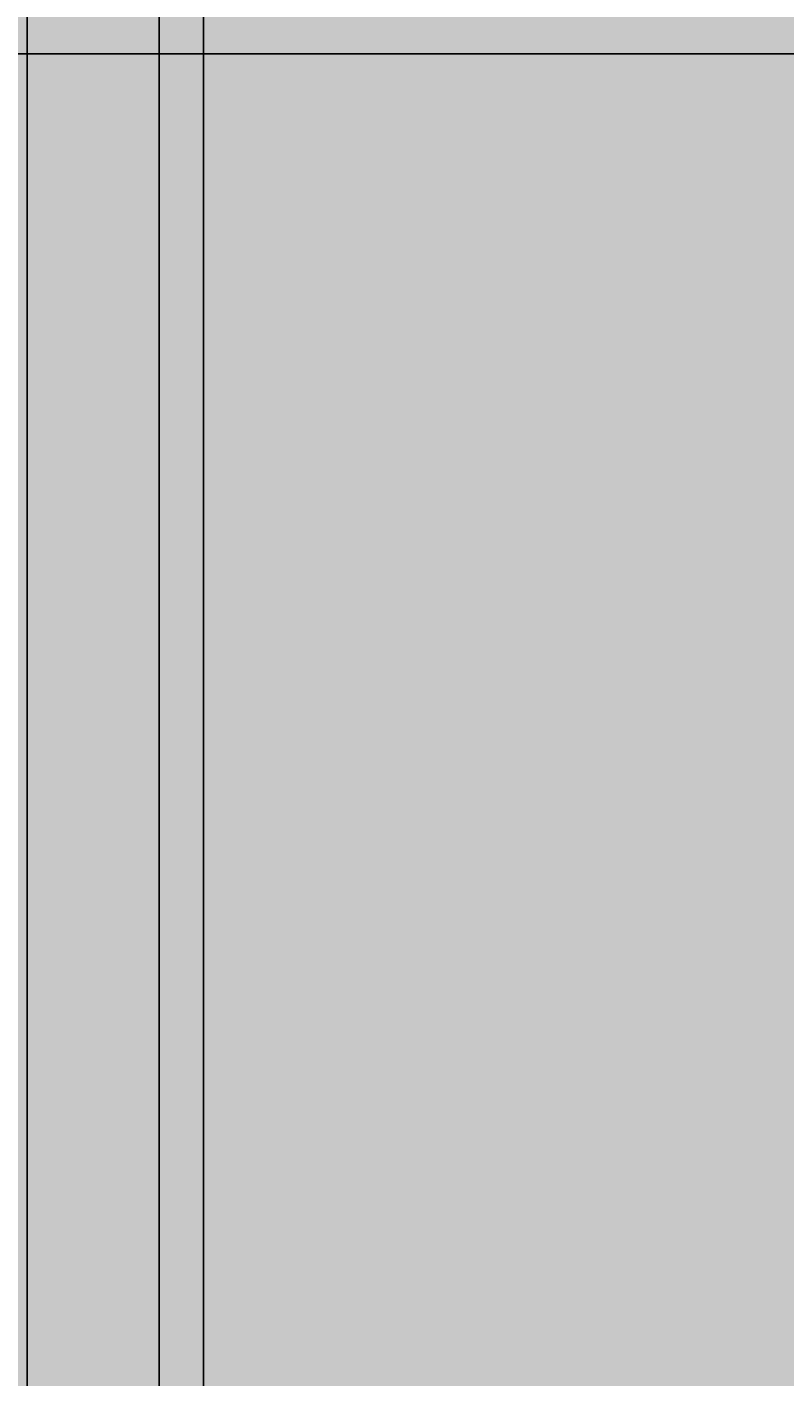
# Model space of a CAD drawing. Units: feet. Extents: x 2695 to 2912, y 795 to 1139.
# Tile 21 of 83: x 2774 to 2791, y 845 to 875. Entities that reach past the tile are written whole.
import ezdxf

# ---------------------------------------------------------------- set-up
doc = ezdxf.new("R2010")
doc.units = ezdxf.units.FT
for name, color, linetype, lineweight in [('A-ANNO-DIMS', 2, 'Continuous', 18), ('A-DOOR', 3, 'Continuous', 25), ('A-DOOR-PATT', 33, 'Continuous', 13), ('A-ELEV-PATT', 252, 'Continuous', 13)]:
    doc.layers.add(name, color=color, linetype=linetype, lineweight=lineweight)
doc.styles.get("Standard").update_dxf_attribs({"font": 'arial.ttf'})
doc.dimstyles.get("Standard").update_dxf_attribs({"dimtxt": 0.18, "dimasz": 0.18, "dimexe": 0.18, "dimexo": 0.0625, "dimgap": 0.09, "dimtad": 0, "dimtih": 1, "dimtoh": 1, "dimdec": 1, "dimzin": 0, "dimdsep": 46, "dimlunit": 3, "dimtxsty": 'Standard', "dimcen": 0.09, "dimadec": 0, "dimazin": 0, "dimtfac": 1, "dimtdec": 1, "dimtofl": 0, "dimtmove": 0, "dimatfit": 3, "dimfxl": 1, "dimtolj": 1, "dimtzin": 0, "dimarcsym": 0})

# ---------------------------------------------------------------- blocks, each defined once
blk = doc.blocks.new('*D13')
at = {"layer": 'A-ANNO-DIMS', "color": 0, "lineweight": -2, "transparency": 16777216}
for p, q in [((2758.214, 874.857), (2911.424, 874.857)), ((2911.244, 874.677), (2911.244, 843.076)), ((2911.244, 811.111), (2911.244, 842.712)), ((2890.699, 810.931), (2911.424, 810.931))]:
    blk.add_line(p, q, dxfattribs=at)
at = {"layer": 'A-ANNO-DIMS', "color": 0, "transparency": 16777216}
for points in [[(2911.214, 874.677), (2911.274, 874.677), (2911.244, 874.857)], [(2911.214, 811.111), (2911.274, 811.111), (2911.244, 810.931)]]:
    blk.add_solid(points, dxfattribs=at)
at = {"layer": 'Defpoints', "color": 0, "transparency": 16777216}
for p in [(2758.151, 874.857), (2911.244, 874.857), (2890.636, 810.931)]:
    blk.add_point(p, dxfattribs=at)
at = {"layer": 'A-ANNO-DIMS', "color": 0, "transparency": 16777216, "insert": (2911.244, 842.894), "char_height": 0.18, "attachment_point": 5}
blk.add_mtext('\\A1;63.93', dxfattribs=at)
blk = doc.blocks.new('*D14')
at = {"layer": 'A-ANNO-DIMS', "color": 0, "lineweight": -2, "transparency": 16777216}
for p, q in [((2838.439, 905.514), (2911.424, 905.514)), ((2911.244, 905.334), (2911.244, 890.368)), ((2911.244, 875.037), (2911.244, 890.004)), ((2758.214, 874.857), (2911.424, 874.857))]:
    blk.add_line(p, q, dxfattribs=at)
at = {"layer": 'A-ANNO-DIMS', "color": 0, "transparency": 16777216}
for points in [[(2911.214, 905.334), (2911.274, 905.334), (2911.244, 905.514)], [(2911.214, 875.037), (2911.274, 875.037), (2911.244, 874.857)]]:
    blk.add_solid(points, dxfattribs=at)
at = {"layer": 'Defpoints', "color": 0, "transparency": 16777216}
for p in [(2838.377, 905.514), (2911.244, 905.514), (2758.151, 874.857)]:
    blk.add_point(p, dxfattribs=at)
at = {"layer": 'A-ANNO-DIMS', "color": 0, "transparency": 16777216, "insert": (2911.244, 890.186), "char_height": 0.18, "attachment_point": 5}
blk.add_mtext('\\A1;30.66', dxfattribs=at)

msp = doc.modelspace()

# ---------------------------------------------------------------- hatches: boundary and pattern name
at = {"layer": 'A-DOOR-PATT'}
h = msp.add_hatch(color=256, dxfattribs=at)
h.set_gradient(color1=(211, 185, 150), color2=(211, 185, 150))
h.paths.add_polyline_path([(2805.9398, 905.5143), (2773.5029, 905.5143), (2773.5029, 810.9306), (2776.4999, 810.9306), (2776.4999, 902.5174), (2802.9429, 902.5174), (2802.9429, 810.9306), (2805.9398, 810.9306)])
h.paths.add_polyline_path([(2803.9681, 874.1057), (2805.0538, 874.1057), (2805.0538, 846.2857), (2803.9681, 846.2857)], flags=16)
h.paths.add_polyline_path([(2838.3767, 905.5143), (2805.9398, 905.5143), (2805.9398, 810.9306), (2808.9368, 810.9306), (2808.9368, 902.5174), (2835.3798, 902.5174), (2835.3798, 810.9306), (2838.3767, 810.9306)])
h = msp.add_hatch(color=256, dxfattribs=at)
h.set_gradient(color1=(211, 185, 150), color2=(211, 185, 150))
h.paths.add_polyline_path([(2777.5029, 901.5143), (2801.9398, 901.5143), (2801.9398, 810.9306), (2802.9429, 810.9306), (2802.9429, 902.5174), (2776.4999, 902.5174), (2776.4999, 810.9306), (2777.5029, 810.9306)])
h.paths.add_polyline_path([(2809.9398, 901.5143), (2834.3767, 901.5143), (2834.3767, 810.9306), (2835.3798, 810.9306), (2835.3798, 902.5174), (2808.9368, 902.5174), (2808.9368, 810.9306), (2809.9398, 810.9306)])
h = msp.add_hatch(color=256, dxfattribs=at)
h.set_gradient(color1=(173, 221, 247), color2=(173, 221, 247))
h.paths.add_polyline_path([(2801.9398, 901.5143), (2777.5029, 901.5143), (2777.5029, 810.9306), (2801.9398, 810.9306)])
h.paths.add_polyline_path([(2834.3767, 901.5143), (2809.9398, 901.5143), (2809.9398, 810.9306), (2834.3767, 810.9306)])
at = {"layer": 'A-ELEV-PATT'}
h = msp.add_hatch(color=256, dxfattribs=at)
h.set_gradient(color1=(147, 149, 152), color2=(147, 149, 152), tint=1)
h.paths.add_polyline_path([(2770.6361, 1118.4096), (2710.6361, 1118.4096), (2710.6361, 1062.9306), (2770.6361, 1062.9306)])
h.paths.add_polyline_path([(2890.6361, 1103.3378), (2770.6361, 1103.3378), (2770.6361, 1062.9306), (2890.6361, 1062.9306)])
h.paths.add_polyline_path([(2730.7081, 1048.1052), (2755.1125, 1048.1052), (2755.1125, 936.9306), (2770.6361, 936.9306), (2770.6361, 1050.3105), (2715.8852, 1050.3105), (2715.8852, 936.9306), (2730.7081, 936.9306)])
h.paths.add_polyline_path([(2890.6361, 1050.3105), (2770.6361, 1050.3105), (2770.6361, 971.9673), (2778.0341, 971.9673), (2778.0341, 1020.8235), (2843.575, 1020.8235), (2843.575, 971.9673), (2890.6361, 971.9673)])
h.paths.add_polyline_path([(2888.1882, 970.7156), (2843.575, 970.7156), (2843.575, 964.8267), (2888.1882, 964.8267)])
h.paths.add_polyline_path([(2888.1882, 964.1328), (2843.575, 964.1328), (2843.575, 956.614), (2888.1882, 956.614)])
h.paths.add_polyline_path([(2888.1882, 955.9202), (2843.575, 955.9202), (2843.575, 949.2892), (2888.1882, 949.2892)])
h.paths.add_polyline_path([(2888.1882, 948.5954), (2843.575, 948.5954), (2843.575, 941.3507), (2888.1882, 941.3507)])
h.paths.add_polyline_path([(2888.1882, 940.6569), (2843.575, 940.6569), (2843.575, 936.9306), (2888.1882, 936.9306)])
h.paths.add_polyline_path([(2890.6361, 970.7156), (2888.9368, 970.7156), (2888.9368, 964.8267), (2890.6361, 964.8267)])
h.paths.add_polyline_path([(2890.6361, 964.1328), (2888.9368, 964.1328), (2888.9368, 956.614), (2890.6361, 956.614)])
h.paths.add_polyline_path([(2890.6361, 955.9202), (2888.9368, 955.9202), (2888.9368, 949.2892), (2890.6361, 949.2892)])
h.paths.add_polyline_path([(2890.6361, 940.6569), (2888.9368, 940.6569), (2888.9368, 936.9306), (2890.6361, 936.9306)])
h.paths.add_polyline_path([(2890.6361, 948.5954), (2888.9368, 948.5954), (2888.9368, 941.3507), (2890.6361, 941.3507)])
h.paths.add_polyline_path([(2772.5216, 970.7156), (2770.6361, 970.7156), (2770.6361, 964.8267), (2772.5216, 964.8267)])
h.paths.add_polyline_path([(2772.5216, 964.1328), (2770.6361, 964.1328), (2770.6361, 956.614), (2772.5216, 956.614)])
h.paths.add_polyline_path([(2772.5216, 955.9202), (2770.6361, 955.9202), (2770.6361, 949.2892), (2772.5216, 949.2892)])
h.paths.add_polyline_path([(2772.5216, 948.5954), (2770.6361, 948.5954), (2770.6361, 941.3507), (2772.5216, 941.3507)])
h.paths.add_polyline_path([(2772.5216, 940.6569), (2770.6361, 940.6569), (2770.6361, 936.9306), (2772.5216, 936.9306)])
h.paths.add_polyline_path([(2778.0341, 940.6569), (2773.2702, 940.6569), (2773.2702, 936.9306), (2778.0341, 936.9306)])
h.paths.add_polyline_path([(2778.0341, 970.7156), (2773.2702, 970.7156), (2773.2702, 964.8267), (2778.0341, 964.8267)])
h.paths.add_polyline_path([(2778.0341, 964.1328), (2773.2702, 964.1328), (2773.2702, 956.614), (2778.0341, 956.614)])
h.paths.add_polyline_path([(2778.0341, 955.9202), (2773.2702, 955.9202), (2773.2702, 949.2892), (2778.0341, 949.2892)])
h.paths.add_polyline_path([(2778.0341, 948.5954), (2773.2702, 948.5954), (2773.2702, 941.3507), (2778.0341, 941.3507)])
h.paths.add_polyline_path([(2810.0407, 940.6569), (2780.0341, 940.6569), (2780.0341, 936.9306), (2810.0407, 936.9306)])
h.paths.add_polyline_path([(2890.6361, 924.3105), (2770.6361, 924.3105), (2770.6361, 810.9306), (2773.5029, 810.9306), (2773.5029, 905.5143), (2805.9398, 905.5143), (2838.3767, 905.5143), (2838.3767, 810.9306), (2890.6361, 810.9306)])

# ---------------------------------------------------------------- linework, layer by layer
at = {"layer": 'A-DOOR'}
for points in [[(2773.5029, 810.9306), (2773.5029, 905.5143), (2805.9398, 905.5143), (2805.9398, 810.9306)], [(2776.4999, 810.9306), (2776.4999, 902.5174), (2802.9429, 902.5174), (2802.9429, 810.9306)], [(2777.5029, 810.9306), (2777.5029, 901.5143), (2801.9398, 901.5143), (2801.9398, 810.9306)]]:
    msp.add_lwpolyline(points, dxfattribs=at)
for points in [[(2773.5029, 905.5143), (2838.3767, 905.5143), (2838.3767, 810.9306), (2773.5029, 810.9306)], [(2776.4999, 902.5174), (2803.0393, 902.5174), (2803.0393, 810.9306), (2776.4999, 810.9306)], [(2777.5029, 901.5143), (2801.9398, 901.5143), (2801.9398, 810.9306), (2777.5029, 810.9306)]]:
    msp.add_lwpolyline(points, close=True, dxfattribs=at)

# ---------------------------------------------------------------- dimensions: what is measured, and where the dimension line sits
at = {"layer": 'A-ANNO-DIMS'}
for base, p1, p2, picture, middle in [((2911.2444, 905.5143), (2758.1515, 874.8571), (2838.3767, 905.5143), '*D14', (2911.2444, 890.1857)), ((2911.2444, 874.8571), (2890.6361, 810.9306), (2758.1515, 874.8571), '*D13', (2911.2444, 842.8938))]:
    dim = msp.add_linear_dim(base=base, p1=p1, p2=p2, angle=90, dimstyle='Standard', override={"dimdec": 2, "dimlfac": 1, "dimrnd": 0, "dimzin": 0, "dimdsep": 46, "dimlunit": 2}, dxfattribs=at)
    dim.commit()
    dim.dimension.update_dxf_attribs({"geometry": picture, "text_midpoint": middle})

doc.saveas('drawing.dxf')
